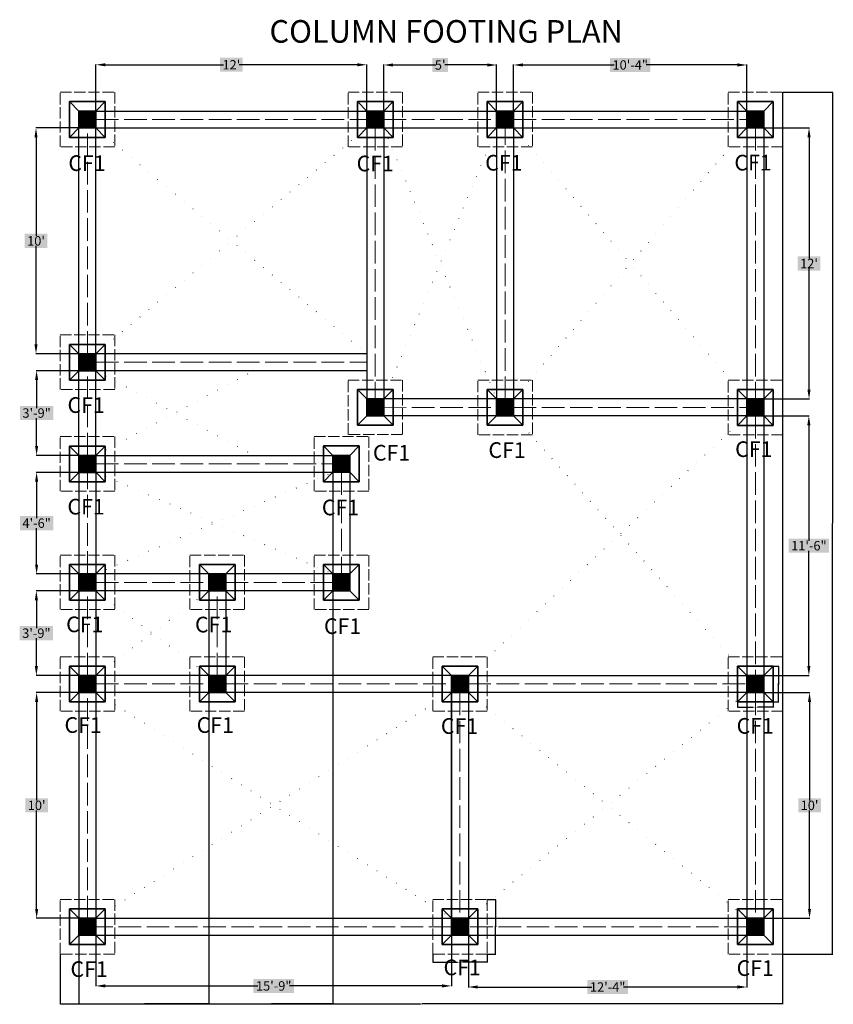
# Model space of a CAD drawing. Units: inches. Extents: x -128 to 854, y -395 to 398.
# Tile 61 of 61: x 395 to 828, y -125 to 398. Entities that reach past the tile are written whole.
import ezdxf

# ---------------------------------------------------------------- set-up
doc = ezdxf.new("R2010")
doc.units = ezdxf.units.IN
doc.header["$MEASUREMENT"] = 0
doc.linetypes.add('ACAD_ISO02W100', pattern=[15, 12, -3])
doc.linetypes.add('ACAD_ISO07W100', pattern=[3, 0, -3])
for name, color, linetype, lineweight in [('A-ANNO-DIMS', 2, 'Continuous', 18), ('A-ANNO-TITL', 7, 'Continuous', 25), ('S-ANNO-DIMS', 2, 'Continuous', 18), ('S-ANNO-TEXT', 7, 'Continuous', 18), ('S-BEAM', 152, 'Continuous', 30), ('S-BEAM-CNTR', 6, 'ACAD_ISO02W100', 13), ('S-COLS', 7, 'Continuous', 35), ('S-COLS-PATT', 8, 'Continuous', 13), ('S-FNDN', 2, 'Continuous', 35), ('S-FNDN-DIAG', 252, 'ACAD_ISO07W100', 13), ('S-FNDN-HIDN', 3, 'ACAD_ISO02W100', 18)]:
    doc.layers.add(name, color=color, linetype=linetype, lineweight=lineweight)
doc.styles.get("Standard").update_dxf_attribs({"font": 'arial.ttf'})
doc.dimstyles.get("Standard").update_dxf_attribs({"dimtxt": 0.18, "dimasz": 0.18, "dimexe": 0.18, "dimexo": 0.0625, "dimgap": 0.09, "dimtad": 0, "dimtih": 1, "dimtoh": 1, "dimdec": 1, "dimzin": 0, "dimdsep": 46, "dimlunit": 4, "dimtxsty": 'Standard', "dimcen": 0.09, "dimclrd": 1, "dimclre": 2, "dimclrt": 6, "dimadec": 0, "dimazin": 0, "dimtfac": 1, "dimtdec": 1, "dimtofl": 0, "dimtmove": 0, "dimatfit": 3, "dimfxl": 1, "dimtfill": 2, "dimtfillclr": 3, "dimtolj": 1, "dimtzin": 0, "dimarcsym": 0})

# ---------------------------------------------------------------- blocks, each defined once
blk = doc.blocks.new('*D16')
at = {"layer": 'Defpoints', "color": 0, "transparency": 16777216}
for p in [(435.64, -79.2), (624.64, -79.2), (624.64, -115.16)]:
    blk.add_point(p, dxfattribs=at)
at = {"layer": 'S-ANNO-DIMS', "color": 0, "lineweight": -2, "transparency": 16777216}
for p, q in [((435.64, -79.27), (435.64, -115.34)), ((624.64, -79.27), (624.64, -115.34)), ((440.64, -115.16), (521.69, -115.16)), ((619.64, -115.16), (538.58, -115.16))]:
    blk.add_line(p, q, dxfattribs=at)
at = {"layer": 'S-ANNO-DIMS', "color": 0, "transparency": 16777216}
for points in [[(440.64, -114.33), (440.64, -116), (435.64, -115.16)], [(619.64, -114.33), (619.64, -116), (624.64, -115.16)]]:
    blk.add_solid(points, dxfattribs=at)
at = {"layer": 'S-ANNO-DIMS', "color": 0, "transparency": 16777216, "insert": (530.14, -115.16), "char_height": 5, "attachment_point": 5, "bg_fill": 1, "box_fill_scale": 1.25, "bg_fill_color": 3, "bg_fill_transparency": 0}
blk.add_mtext('\\A1;15\'-9"', dxfattribs=at)
blk = doc.blocks.new('*D17')
at = {"layer": 'Defpoints', "color": 0, "transparency": 16777216}
for p in [(633.64, -79.2), (781.64, -79.2), (781.64, -115.74)]:
    blk.add_point(p, dxfattribs=at)
at = {"layer": 'S-ANNO-DIMS', "color": 0, "lineweight": -2, "transparency": 16777216}
for p, q in [((633.64, -79.27), (633.64, -115.92)), ((781.64, -79.27), (781.64, -115.92)), ((638.64, -115.74), (699.19, -115.74)), ((776.64, -115.74), (716.08, -115.74))]:
    blk.add_line(p, q, dxfattribs=at)
at = {"layer": 'S-ANNO-DIMS', "color": 0, "transparency": 16777216}
for points in [[(638.64, -114.9), (638.64, -116.57), (633.64, -115.74)], [(776.64, -114.9), (776.64, -116.57), (781.64, -115.74)]]:
    blk.add_solid(points, dxfattribs=at)
at = {"layer": 'S-ANNO-DIMS', "color": 0, "transparency": 16777216, "insert": (707.64, -115.74), "char_height": 5, "attachment_point": 5, "bg_fill": 1, "box_fill_scale": 1.25, "bg_fill_color": 3, "bg_fill_transparency": 0}
blk.add_mtext('\\A1;12\'-4"', dxfattribs=at)
blk = doc.blocks.new('*D18')
at = {"layer": 'Defpoints', "color": 0, "transparency": 16777216}
for p in [(781.64, 40.8), (814.94, 40.8), (781.64, -79.2)]:
    blk.add_point(p, dxfattribs=at)
at = {"layer": 'S-ANNO-DIMS', "color": 0, "lineweight": -2, "transparency": 16777216}
for p, q in [((781.7, 40.8), (815.12, 40.8)), ((814.94, 35.8), (814.94, -16.56)), ((814.94, -74.2), (814.94, -21.85)), ((781.7, -79.2), (815.12, -79.2))]:
    blk.add_line(p, q, dxfattribs=at)
at = {"layer": 'S-ANNO-DIMS', "color": 0, "transparency": 16777216}
for points in [[(814.1, 35.8), (815.77, 35.8), (814.94, 40.8)], [(814.1, -74.2), (815.77, -74.2), (814.94, -79.2)]]:
    blk.add_solid(points, dxfattribs=at)
at = {"layer": 'S-ANNO-DIMS', "color": 0, "transparency": 16777216, "insert": (814.94, -19.2), "char_height": 5, "attachment_point": 5, "bg_fill": 1, "box_fill_scale": 1.25, "bg_fill_color": 3, "bg_fill_transparency": 0}
blk.add_mtext("\\A1;10'", dxfattribs=at)
blk = doc.blocks.new('*D19')
at = {"layer": 'Defpoints', "color": 0, "transparency": 16777216}
for p in [(781.64, 187.8), (814.59, 187.8), (781.64, 49.8)]:
    blk.add_point(p, dxfattribs=at)
at = {"layer": 'S-ANNO-DIMS', "color": 0, "lineweight": -2, "transparency": 16777216}
for p, q in [((781.7, 187.8), (814.77, 187.8)), ((781.7, 49.8), (814.77, 49.8))]:
    blk.add_line(p, q, dxfattribs=at)
at = {"layer": 'S-ANNO-DIMS', "color": 0, "lineweight": -3, "transparency": 16777216}
for p, q in [((814.59, 182.8), (814.59, 121.44)), ((814.59, 54.8), (814.59, 116.15))]:
    blk.add_line(p, q, dxfattribs=at)
at = {"layer": 'S-ANNO-DIMS', "color": 0, "transparency": 16777216}
for points in [[(813.76, 182.8), (815.42, 182.8), (814.59, 187.8)], [(813.76, 54.8), (815.42, 54.8), (814.59, 49.8)]]:
    blk.add_solid(points, dxfattribs=at)
at = {"layer": 'S-ANNO-DIMS', "color": 0, "transparency": 16777216, "insert": (814.59, 118.8), "char_height": 5, "attachment_point": 5, "bg_fill": 1, "box_fill_scale": 1.25, "bg_fill_color": 3, "bg_fill_transparency": 0}
blk.add_mtext('\\A1;11\'-6"', dxfattribs=at)
blk = doc.blocks.new('*D20')
at = {"layer": 'Defpoints', "color": 0, "transparency": 16777216}
for p in [(781.64, 340.8), (814.67, 340.8), (781.64, 196.76)]:
    blk.add_point(p, dxfattribs=at)
at = {"layer": 'S-ANNO-DIMS', "color": 0, "lineweight": -2, "transparency": 16777216}
for p, q in [((781.7, 340.8), (814.85, 340.8)), ((814.67, 335.8), (814.67, 271.38)), ((814.67, 201.76), (814.67, 266.18)), ((781.7, 196.76), (814.85, 196.76))]:
    blk.add_line(p, q, dxfattribs=at)
at = {"layer": 'S-ANNO-DIMS', "color": 0, "transparency": 16777216}
for points in [[(813.83, 335.8), (815.5, 335.8), (814.67, 340.8)], [(813.83, 201.76), (815.5, 201.76), (814.67, 196.76)]]:
    blk.add_solid(points, dxfattribs=at)
at = {"layer": 'S-ANNO-DIMS', "color": 0, "transparency": 16777216, "insert": (814.67, 268.78), "char_height": 5, "attachment_point": 5, "bg_fill": 1, "box_fill_scale": 1.25, "bg_fill_color": 3, "bg_fill_transparency": 0}
blk.add_mtext("\\A1;12'", dxfattribs=at)
blk = doc.blocks.new('*D21')
at = {"layer": 'Defpoints', "color": 0, "transparency": 16777216}
for p in [(781.64, 374.28), (657.64, 340.8), (781.64, 340.8)]:
    blk.add_point(p, dxfattribs=at)
at = {"layer": 'S-ANNO-DIMS', "color": 0, "lineweight": -2, "transparency": 16777216}
for p, q in [((657.64, 340.86), (657.64, 374.46)), ((662.64, 374.28), (711.19, 374.28)), ((776.64, 374.28), (728.08, 374.28)), ((781.64, 340.86), (781.64, 374.46))]:
    blk.add_line(p, q, dxfattribs=at)
at = {"layer": 'S-ANNO-DIMS', "color": 0, "transparency": 16777216}
for points in [[(662.64, 375.12), (662.64, 373.45), (657.64, 374.28)], [(776.64, 375.12), (776.64, 373.45), (781.64, 374.28)]]:
    blk.add_solid(points, dxfattribs=at)
at = {"layer": 'S-ANNO-DIMS', "color": 0, "transparency": 16777216, "insert": (719.64, 374.28), "char_height": 5, "attachment_point": 5, "bg_fill": 1, "box_fill_scale": 1.25, "bg_fill_color": 3, "bg_fill_transparency": 0}
blk.add_mtext('\\A1;10\'-4"', dxfattribs=at)
blk = doc.blocks.new('*D22')
at = {"layer": 'Defpoints', "color": 0, "transparency": 16777216}
for p in [(648.64, 374.27), (588.64, 340.8), (648.64, 340.8)]:
    blk.add_point(p, dxfattribs=at)
at = {"layer": 'S-ANNO-DIMS', "color": 0, "lineweight": -2, "transparency": 16777216}
for p, q in [((588.64, 340.86), (588.64, 374.45)), ((593.64, 374.27), (616.25, 374.27)), ((643.64, 374.27), (621.03, 374.27)), ((648.64, 340.86), (648.64, 374.45))]:
    blk.add_line(p, q, dxfattribs=at)
at = {"layer": 'S-ANNO-DIMS', "color": 0, "transparency": 16777216}
for points in [[(593.64, 375.1), (593.64, 373.43), (588.64, 374.27)], [(643.64, 375.1), (643.64, 373.43), (648.64, 374.27)]]:
    blk.add_solid(points, dxfattribs=at)
at = {"layer": 'S-ANNO-DIMS', "color": 0, "transparency": 16777216, "insert": (618.64, 374.27), "char_height": 5, "attachment_point": 5, "bg_fill": 1, "box_fill_scale": 1.25, "bg_fill_color": 3, "bg_fill_transparency": 0}
blk.add_mtext("\\A1;5'", dxfattribs=at)
blk = doc.blocks.new('*D23')
at = {"layer": 'Defpoints', "color": 0, "transparency": 16777216}
for p in [(579.64, 374.38), (435.64, 340.8), (579.64, 340.8)]:
    blk.add_point(p, dxfattribs=at)
at = {"layer": 'S-ANNO-DIMS', "color": 0, "lineweight": -2, "transparency": 16777216}
for p, q in [((435.64, 340.86), (435.64, 374.56)), ((440.64, 374.38), (503.54, 374.38)), ((574.64, 374.38), (511.73, 374.38)), ((579.64, 340.86), (579.64, 374.56))]:
    blk.add_line(p, q, dxfattribs=at)
at = {"layer": 'S-ANNO-DIMS', "color": 0, "transparency": 16777216}
for points in [[(440.64, 375.21), (440.64, 373.55), (435.64, 374.38)], [(574.64, 375.21), (574.64, 373.55), (579.64, 374.38)]]:
    blk.add_solid(points, dxfattribs=at)
at = {"layer": 'S-ANNO-DIMS', "color": 0, "transparency": 16777216, "insert": (507.64, 374.38), "char_height": 5, "attachment_point": 5, "bg_fill": 1, "box_fill_scale": 1.25, "bg_fill_color": 3, "bg_fill_transparency": 0}
blk.add_mtext("\\A1;12'", dxfattribs=at)
blk = doc.blocks.new('*D24')
at = {"layer": 'Defpoints', "color": 0, "transparency": 16777216}
for p in [(435.64, 340.8), (403.82, 220.8), (435.64, 220.8)]:
    blk.add_point(p, dxfattribs=at)
at = {"layer": 'S-ANNO-DIMS', "color": 0, "lineweight": -2, "transparency": 16777216}
for p, q in [((435.57, 340.8), (403.64, 340.8)), ((403.82, 335.8), (403.82, 283.44)), ((403.82, 225.8), (403.82, 278.15)), ((435.57, 220.8), (403.64, 220.8))]:
    blk.add_line(p, q, dxfattribs=at)
at = {"layer": 'S-ANNO-DIMS', "color": 0, "transparency": 16777216}
for points in [[(402.99, 335.8), (404.65, 335.8), (403.82, 340.8)], [(402.99, 225.8), (404.65, 225.8), (403.82, 220.8)]]:
    blk.add_solid(points, dxfattribs=at)
at = {"layer": 'S-ANNO-DIMS', "color": 0, "transparency": 16777216, "insert": (403.82, 280.8), "char_height": 5, "attachment_point": 5, "bg_fill": 1, "box_fill_scale": 1.25, "bg_fill_color": 3, "bg_fill_transparency": 0}
blk.add_mtext("\\A1;10'", dxfattribs=at)
blk = doc.blocks.new('*D25')
at = {"layer": 'Defpoints', "color": 0, "transparency": 16777216}
for p in [(435.64, 211.8), (404.14, 166.8), (435.64, 166.8)]:
    blk.add_point(p, dxfattribs=at)
at = {"layer": 'S-ANNO-DIMS', "color": 0, "lineweight": -2, "transparency": 16777216}
for p, q in [((435.57, 211.8), (403.96, 211.8)), ((404.14, 206.8), (404.14, 191.94)), ((404.14, 171.8), (404.14, 186.65)), ((435.57, 166.8), (403.96, 166.8))]:
    blk.add_line(p, q, dxfattribs=at)
at = {"layer": 'S-ANNO-DIMS', "color": 0, "transparency": 16777216}
for points in [[(403.3, 206.8), (404.97, 206.8), (404.14, 211.8)], [(403.3, 171.8), (404.97, 171.8), (404.14, 166.8)]]:
    blk.add_solid(points, dxfattribs=at)
at = {"layer": 'S-ANNO-DIMS', "color": 0, "transparency": 16777216, "insert": (404.14, 189.3), "char_height": 5, "attachment_point": 5, "bg_fill": 1, "box_fill_scale": 1.25, "bg_fill_color": 3, "bg_fill_transparency": 0}
blk.add_mtext('\\A1;3\'-9"', dxfattribs=at)
blk = doc.blocks.new('*D26')
at = {"layer": 'Defpoints', "color": 0, "transparency": 16777216}
for p in [(435.64, 157.76), (404.15, 103.8), (435.64, 103.8)]:
    blk.add_point(p, dxfattribs=at)
at = {"layer": 'S-ANNO-DIMS', "color": 0, "lineweight": -2, "transparency": 16777216}
for p, q in [((435.57, 157.76), (403.97, 157.76)), ((404.15, 152.76), (404.15, 133.42)), ((404.15, 108.8), (404.15, 128.14)), ((435.57, 103.8), (403.97, 103.8))]:
    blk.add_line(p, q, dxfattribs=at)
at = {"layer": 'S-ANNO-DIMS', "color": 0, "transparency": 16777216}
for points in [[(403.31, 152.76), (404.98, 152.76), (404.15, 157.76)], [(403.31, 108.8), (404.98, 108.8), (404.15, 103.8)]]:
    blk.add_solid(points, dxfattribs=at)
at = {"layer": 'S-ANNO-DIMS', "color": 0, "transparency": 16777216, "insert": (404.15, 130.78), "char_height": 5, "attachment_point": 5, "bg_fill": 1, "box_fill_scale": 1.25, "bg_fill_color": 3, "bg_fill_transparency": 0}
blk.add_mtext('\\A1;4\'-6"', dxfattribs=at)
blk = doc.blocks.new('*D27')
at = {"layer": 'Defpoints', "color": 0, "transparency": 16777216}
for p in [(435.64, 94.8), (404.01, 49.8), (435.64, 49.8)]:
    blk.add_point(p, dxfattribs=at)
at = {"layer": 'S-ANNO-DIMS', "color": 0, "lineweight": -2, "transparency": 16777216}
for p, q in [((435.57, 94.8), (403.83, 94.8)), ((404.01, 89.8), (404.01, 74.94)), ((404.01, 54.8), (404.01, 69.65)), ((435.57, 49.8), (403.83, 49.8))]:
    blk.add_line(p, q, dxfattribs=at)
at = {"layer": 'S-ANNO-DIMS', "color": 0, "transparency": 16777216}
for points in [[(403.17, 89.8), (404.84, 89.8), (404.01, 94.8)], [(403.17, 54.8), (404.84, 54.8), (404.01, 49.8)]]:
    blk.add_solid(points, dxfattribs=at)
at = {"layer": 'S-ANNO-DIMS', "color": 0, "transparency": 16777216, "insert": (404.01, 72.3), "char_height": 5, "attachment_point": 5, "bg_fill": 1, "box_fill_scale": 1.25, "bg_fill_color": 3, "bg_fill_transparency": 0}
blk.add_mtext('\\A1;3\'-9"', dxfattribs=at)
blk = doc.blocks.new('*D28')
at = {"layer": 'Defpoints', "color": 0, "transparency": 16777216}
for p in [(404.16, 40.8), (435.64, 40.8), (435.64, -79.2)]:
    blk.add_point(p, dxfattribs=at)
at = {"layer": 'S-ANNO-DIMS', "color": 0, "lineweight": -2, "transparency": 16777216}
for p, q in [((435.57, 40.8), (403.98, 40.8)), ((404.16, 35.8), (404.16, -16.56)), ((404.16, -74.2), (404.16, -21.85)), ((435.57, -79.2), (403.98, -79.2))]:
    blk.add_line(p, q, dxfattribs=at)
at = {"layer": 'S-ANNO-DIMS', "color": 0, "transparency": 16777216}
for points in [[(403.33, 35.8), (405, 35.8), (404.16, 40.8)], [(403.33, -74.2), (405, -74.2), (404.16, -79.2)]]:
    blk.add_solid(points, dxfattribs=at)
at = {"layer": 'S-ANNO-DIMS', "color": 0, "transparency": 16777216, "insert": (404.16, -19.2), "char_height": 5, "attachment_point": 5, "bg_fill": 1, "box_fill_scale": 1.25, "bg_fill_color": 3, "bg_fill_transparency": 0}
blk.add_mtext("\\A1;10'", dxfattribs=at)
blk = doc.blocks.new('CF1-BASE-29IN')
at = {"ltscale": 0.5}
for p, q in [((0, 29), (29, 29)), ((0, 0), (0, 29)), ((29, 29), (29, 0)), ((29, 0), (0, 0))]:
    blk.add_line(p, q, dxfattribs=at)
blk = doc.blocks.new('CF1-PAD-19IN')
for p, q in [((0, 19), (19, 19)), ((0, 0), (0, 19)), ((19, 19), (19, 0)), ((19, 0), (0, 0))]:
    blk.add_line(p, q)
blk = doc.blocks.new('*D67')
at = {"layer": 'A-ANNO-DIMS', "color": 2, "lineweight": -2, "transparency": 16777216}
for p, q in [((614.64, -98.27), (614.64, -102.73)), ((643.64, -98.27), (643.64, -102.73))]:
    blk.add_line(p, q, dxfattribs=at)
at = {"layer": 'A-ANNO-DIMS', "color": 1, "lineweight": -2, "transparency": 16777216}
for p, q in [((614.82, -102.55), (627.86, -102.55)), ((643.46, -102.55), (630.42, -102.55))]:
    blk.add_line(p, q, dxfattribs=at)
at = {"layer": 'A-ANNO-DIMS', "color": 1, "transparency": 16777216}
for points in [[(614.82, -102.52), (614.82, -102.58), (614.64, -102.55)], [(643.46, -102.52), (643.46, -102.58), (643.64, -102.55)]]:
    blk.add_solid(points, dxfattribs=at)
at = {"layer": 'Defpoints', "color": 0, "transparency": 16777216}
for p in [(614.64, -98.2), (643.64, -98.2), (643.64, -102.55)]:
    blk.add_point(p, dxfattribs=at)
at = {"layer": 'A-ANNO-DIMS', "color": 6, "transparency": 16777216, "insert": (629.14, -102.55), "char_height": 0.18, "attachment_point": 5, "bg_fill": 1, "box_fill_scale": 1.25, "bg_fill_color": 3, "bg_fill_transparency": 0}
blk.add_mtext('\\A1;CF1 BASE 2\'-5" TYP.', dxfattribs=at)
blk = doc.blocks.new('*D68')
at = {"layer": 'A-ANNO-DIMS', "color": 2, "lineweight": -2, "transparency": 16777216}
for p, q in [((643.7, -69.2), (648.17, -69.2)), ((643.7, -98.2), (648.17, -98.2))]:
    blk.add_line(p, q, dxfattribs=at)
at = {"layer": 'A-ANNO-DIMS', "color": 1, "lineweight": -2, "transparency": 16777216}
for p, q in [((647.99, -69.38), (647.99, -83.52)), ((647.99, -98.02), (647.99, -83.88))]:
    blk.add_line(p, q, dxfattribs=at)
at = {"layer": 'A-ANNO-DIMS', "color": 1, "transparency": 16777216}
for points in [[(647.96, -69.38), (648.02, -69.38), (647.99, -69.2)], [(647.96, -98.02), (648.02, -98.02), (647.99, -98.2)]]:
    blk.add_solid(points, dxfattribs=at)
at = {"layer": 'Defpoints', "color": 0, "transparency": 16777216}
for p in [(643.64, -69.2), (647.99, -69.2), (643.64, -98.2)]:
    blk.add_point(p, dxfattribs=at)
at = {"layer": 'A-ANNO-DIMS', "color": 6, "transparency": 16777216, "insert": (647.99, -83.7), "char_height": 0.18, "attachment_point": 5, "bg_fill": 1, "box_fill_scale": 1.25, "bg_fill_color": 3, "bg_fill_transparency": 0}
blk.add_mtext('\\A1;2\'-5" TYP.', dxfattribs=at)
blk = doc.blocks.new('*D69')
at = {"layer": 'A-ANNO-DIMS', "color": 2, "lineweight": -2, "transparency": 16777216}
for p, q in [((776.64, 35.73), (776.64, 32.77)), ((795.64, 35.73), (795.64, 32.77))]:
    blk.add_line(p, q, dxfattribs=at)
at = {"layer": 'A-ANNO-DIMS', "color": 1, "lineweight": -2, "transparency": 16777216}
for p, q in [((776.82, 32.95), (784.93, 32.95)), ((795.46, 32.95), (787.34, 32.95))]:
    blk.add_line(p, q, dxfattribs=at)
at = {"layer": 'A-ANNO-DIMS', "color": 1, "transparency": 16777216}
for points in [[(776.82, 32.98), (776.82, 32.92), (776.64, 32.95)], [(795.46, 32.98), (795.46, 32.92), (795.64, 32.95)]]:
    blk.add_solid(points, dxfattribs=at)
at = {"layer": 'Defpoints', "color": 0, "transparency": 16777216}
for p in [(776.64, 35.8), (795.64, 35.8), (795.64, 32.95)]:
    blk.add_point(p, dxfattribs=at)
at = {"layer": 'A-ANNO-DIMS', "color": 6, "transparency": 16777216, "insert": (786.14, 32.95), "char_height": 0.18, "attachment_point": 5, "bg_fill": 1, "box_fill_scale": 1.25, "bg_fill_color": 3, "bg_fill_transparency": 0}
blk.add_mtext('\\A1;CF1 PAD 1\'-7" TYP.', dxfattribs=at)
blk = doc.blocks.new('*D70')
at = {"layer": 'A-ANNO-DIMS', "color": 2, "lineweight": -2, "transparency": 16777216}
for p, q in [((795.7, 54.8), (798.67, 54.8)), ((795.7, 35.8), (798.67, 35.8))]:
    blk.add_line(p, q, dxfattribs=at)
at = {"layer": 'A-ANNO-DIMS', "color": 1, "lineweight": -2, "transparency": 16777216}
for p, q in [((798.49, 54.62), (798.49, 45.48)), ((798.49, 35.98), (798.49, 45.12))]:
    blk.add_line(p, q, dxfattribs=at)
at = {"layer": 'A-ANNO-DIMS', "color": 1, "transparency": 16777216}
for points in [[(798.46, 54.62), (798.52, 54.62), (798.49, 54.8)], [(798.46, 35.98), (798.52, 35.98), (798.49, 35.8)]]:
    blk.add_solid(points, dxfattribs=at)
at = {"layer": 'Defpoints', "color": 0, "transparency": 16777216}
for p in [(795.64, 54.8), (798.49, 54.8), (795.64, 35.8)]:
    blk.add_point(p, dxfattribs=at)
at = {"layer": 'A-ANNO-DIMS', "color": 6, "transparency": 16777216, "insert": (798.49, 45.3), "char_height": 0.18, "attachment_point": 5, "bg_fill": 1, "box_fill_scale": 1.25, "bg_fill_color": 3, "bg_fill_transparency": 0}
blk.add_mtext('\\A1;1\'-7" TYP.', dxfattribs=at)
blk = doc.blocks.new('*D115')
at = {"layer": 'A-ANNO-DIMS', "color": 2, "lineweight": -2, "transparency": 16777216}
for p, q in [((800.64, 359.73), (800.64, -124.93)), ((416.64, -98.27), (416.64, -124.93))]:
    blk.add_line(p, q, dxfattribs=at)
at = {"layer": 'A-ANNO-DIMS', "color": 1, "lineweight": -2, "transparency": 16777216}
for p, q in [((416.82, -124.75), (608.24, -124.75)), ((800.46, -124.75), (609.04, -124.75))]:
    blk.add_line(p, q, dxfattribs=at)
at = {"layer": 'A-ANNO-DIMS', "color": 1, "transparency": 16777216}
for points in [[(416.82, -124.72), (416.82, -124.78), (416.64, -124.75)], [(800.46, -124.72), (800.46, -124.78), (800.64, -124.75)]]:
    blk.add_solid(points, dxfattribs=at)
at = {"layer": 'Defpoints', "color": 0, "transparency": 16777216}
for p in [(800.64, 359.8), (416.64, -98.2), (800.64, -124.75)]:
    blk.add_point(p, dxfattribs=at)
at = {"layer": 'A-ANNO-DIMS', "color": 6, "transparency": 16777216, "insert": (608.64, -124.75), "char_height": 0.18, "attachment_point": 5, "bg_fill": 1, "box_fill_scale": 1.25, "bg_fill_color": 3, "bg_fill_transparency": 0}
blk.add_mtext('\\A1;32\'-0"', dxfattribs=at)
blk = doc.blocks.new('*D116')
at = {"layer": 'A-ANNO-DIMS', "color": 2, "lineweight": -2, "transparency": 16777216}
for p, q in [((800.7, 359.8), (827.37, 359.8)), ((800.7, -98.2), (827.37, -98.2))]:
    blk.add_line(p, q, dxfattribs=at)
at = {"layer": 'A-ANNO-DIMS', "color": 1, "lineweight": -2, "transparency": 16777216}
for p, q in [((827.19, 359.62), (827.19, 130.98)), ((827.19, -98.02), (827.19, 130.62))]:
    blk.add_line(p, q, dxfattribs=at)
at = {"layer": 'A-ANNO-DIMS', "color": 1, "transparency": 16777216}
for points in [[(827.16, 359.62), (827.22, 359.62), (827.19, 359.8)], [(827.16, -98.02), (827.22, -98.02), (827.19, -98.2)]]:
    blk.add_solid(points, dxfattribs=at)
at = {"layer": 'Defpoints', "color": 0, "transparency": 16777216}
for p in [(800.64, 359.8), (827.19, 359.8), (800.64, -98.2)]:
    blk.add_point(p, dxfattribs=at)
at = {"layer": 'A-ANNO-DIMS', "color": 6, "transparency": 16777216, "insert": (827.19, 130.8), "char_height": 0.18, "attachment_point": 5, "bg_fill": 1, "box_fill_scale": 1.25, "bg_fill_color": 3, "bg_fill_transparency": 0}
blk.add_mtext('\\A1;38\'-2"', dxfattribs=at)
blk = doc.blocks.new('*D117')
at = {"layer": 'A-ANNO-DIMS', "color": 2, "lineweight": -2, "transparency": 16777216}
for p, q in [((426.64, 103.73), (426.64, -124.93)), ((495.64, 103.73), (495.64, -124.93))]:
    blk.add_line(p, q, dxfattribs=at)
at = {"layer": 'A-ANNO-DIMS', "color": 1, "lineweight": -2, "transparency": 16777216}
for p, q in [((426.82, -124.75), (460.81, -124.75)), ((495.46, -124.75), (461.47, -124.75))]:
    blk.add_line(p, q, dxfattribs=at)
at = {"layer": 'A-ANNO-DIMS', "color": 1, "transparency": 16777216}
for points in [[(426.82, -124.72), (426.82, -124.78), (426.64, -124.75)], [(495.46, -124.72), (495.46, -124.78), (495.64, -124.75)]]:
    blk.add_solid(points, dxfattribs=at)
at = {"layer": 'Defpoints', "color": 0, "transparency": 16777216}
for p in [(426.64, 103.8), (495.64, 103.8), (495.64, -124.75)]:
    blk.add_point(p, dxfattribs=at)
at = {"layer": 'A-ANNO-DIMS', "color": 6, "transparency": 16777216, "insert": (461.14, -124.75), "char_height": 0.18, "attachment_point": 5, "bg_fill": 1, "box_fill_scale": 1.25, "bg_fill_color": 3, "bg_fill_transparency": 0}
blk.add_mtext('\\A1;5\'-9"', dxfattribs=at)
blk = doc.blocks.new('*D118')
at = {"layer": 'A-ANNO-DIMS', "color": 2, "lineweight": -2, "transparency": 16777216}
for p, q in [((495.64, 103.73), (495.64, -124.93)), ((561.64, 103.73), (561.64, -124.93))]:
    blk.add_line(p, q, dxfattribs=at)
at = {"layer": 'A-ANNO-DIMS', "color": 1, "lineweight": -2, "transparency": 16777216}
for p, q in [((495.82, -124.75), (528.31, -124.75)), ((561.46, -124.75), (528.97, -124.75))]:
    blk.add_line(p, q, dxfattribs=at)
at = {"layer": 'A-ANNO-DIMS', "color": 1, "transparency": 16777216}
for points in [[(495.82, -124.72), (495.82, -124.78), (495.64, -124.75)], [(561.46, -124.72), (561.46, -124.78), (561.64, -124.75)]]:
    blk.add_solid(points, dxfattribs=at)
at = {"layer": 'Defpoints', "color": 0, "transparency": 16777216}
for p in [(495.64, 103.8), (561.64, 103.8), (561.64, -124.75)]:
    blk.add_point(p, dxfattribs=at)
at = {"layer": 'A-ANNO-DIMS', "color": 6, "transparency": 16777216, "insert": (528.64, -124.75), "char_height": 0.18, "attachment_point": 5, "bg_fill": 1, "box_fill_scale": 1.25, "bg_fill_color": 3, "bg_fill_transparency": 0}
blk.add_mtext('\\A1;5\'-6"', dxfattribs=at)

msp = doc.modelspace()

# ---------------------------------------------------------------- hatches: boundary and pattern name
at = {"layer": 'S-COLS-PATT'}
h = msp.add_hatch(dxfattribs=at)
h.set_pattern_fill('ANSI31', color=256)
h.paths.add_polyline_path([(435.64, 349.8), (426.64, 349.8), (426.64, 340.8), (435.64, 340.8)])
h.paths.add_polyline_path([(588.64, 349.8), (579.64, 349.8), (579.64, 340.8), (588.64, 340.8)])
h.paths.add_polyline_path([(657.64, 349.8), (648.64, 349.8), (648.64, 340.8), (657.64, 340.8)])
h.paths.add_polyline_path([(790.64, 349.8), (781.64, 349.8), (781.64, 340.8), (790.64, 340.8)])
h.paths.add_polyline_path([(435.64, 220.8), (426.64, 220.8), (426.64, 211.8), (435.64, 211.8)])
h.paths.add_polyline_path([(588.64, 196.8), (579.64, 196.8), (579.64, 187.83), (588.64, 187.83)])
h.paths.add_polyline_path([(657.64, 196.8), (648.64, 196.8), (648.64, 187.8), (657.64, 187.8)])
h.paths.add_polyline_path([(790.64, 196.76), (781.64, 196.76), (781.64, 187.76), (790.64, 187.76)])
h.paths.add_polyline_path([(435.64, 166.76), (426.64, 166.76), (426.64, 157.76), (435.64, 157.76)])
h.paths.add_polyline_path([(570.64, 166.8), (561.64, 166.8), (561.64, 157.8), (570.64, 157.8)])
h.paths.add_polyline_path([(435.64, 103.8), (426.64, 103.8), (426.64, 94.8), (435.64, 94.8)])
h.paths.add_polyline_path([(504.64, 103.8), (495.64, 103.8), (495.64, 94.8), (504.64, 94.8)])
h.paths.add_polyline_path([(570.64, 103.8), (561.64, 103.8), (561.64, 94.8), (570.64, 94.8)])
h.paths.add_polyline_path([(435.64, 49.8), (426.64, 49.8), (426.64, 40.8), (435.64, 40.8)])
h.paths.add_polyline_path([(504.64, 49.8), (495.64, 49.8), (495.64, 40.8), (504.64, 40.8)])
h.paths.add_polyline_path([(633.64, 49.8), (624.64, 49.8), (624.64, 40.8), (633.64, 40.8)])
h.paths.add_polyline_path([(790.64, 49.8), (781.64, 49.8), (781.64, 40.8), (790.64, 40.8)])
h.paths.add_polyline_path([(435.64, -79.2), (426.64, -79.2), (426.64, -88.2), (435.64, -88.2)])
h.paths.add_polyline_path([(633.64, -79.2), (624.64, -79.2), (624.64, -88.2), (633.64, -88.2)])
h.paths.add_polyline_path([(790.64, -79.2), (781.64, -79.2), (781.64, -88.2), (790.64, -88.2)])

# ---------------------------------------------------------------- linework, layer by layer
at = {"layer": 'S-BEAM'}
for p, q in [((426.64, 162.3), (426.64, 349.8)), ((426.64, 349.8), (790.64, 349.8)), ((790.64, 349.8), (790.64, -88.2)), ((435.64, 220.8), (435.64, 340.8)), ((435.64, 340.8), (579.64, 340.8)), ((579.64, 340.8), (579.64, 187.8)), ((588.64, 340.8), (588.64, 187.8)), ((588.64, 340.8), (648.64, 340.8)), ((648.64, 340.8), (648.64, 220.8)), ((648.64, 340.8), (648.64, 196.83)), ((657.64, 340.8), (657.64, 196.8)), ((657.64, 340.8), (781.64, 340.8)), ((781.64, 340.8), (781.64, 196.8)), ((579.64, 220.8), (435.64, 220.8)), ((579.64, 211.8), (426.64, 211.8)), ((435.64, 166.8), (435.64, 211.8)), ((781.64, 196.8), (579.64, 196.8)), ((781.64, 187.8), (579.64, 187.8)), ((781.64, 187.8), (781.64, 73.8)), ((426.64, 166.8), (570.64, 166.8)), ((570.64, 166.8), (570.64, 94.8)), ((426.64, 161.98), (426.64, 94.8)), ((435.64, 157.8), (435.64, 103.8)), ((435.64, 157.8), (561.64, 157.8)), ((561.64, 157.8), (561.64, 103.8)), ((435.64, 103.8), (435.64, 49.8)), ((561.64, 103.8), (435.64, 103.8)), ((426.64, 94.8), (426.64, 40.8)), ((570.64, 94.8), (435.64, 94.8)), ((495.64, 94.8), (495.64, 49.8)), ((504.64, 94.8), (504.64, 49.8)), ((781.64, 84.8), (781.64, -79.2)), ((495.64, 49.8), (435.64, 49.8)), ((633.64, 49.8), (504.64, 49.8)), ((633.64, 49.8), (633.64, -79.2)), ((633.64, 49.8), (790.64, 49.8)), ((426.64, 40.8), (426.64, -88.2)), ((519.64, 40.8), (435.64, 40.8)), ((435.64, 40.8), (435.64, -79.2)), ((790.64, 40.8), (495.64, 40.8)), ((624.64, -79.2), (624.64, 40.8)), ((624.64, 40.8), (624.64, -79.2)), ((435.64, -79.2), (561.64, -79.2)), ((559.66, -79.2), (624.64, -79.2)), ((633.64, -79.2), (781.64, -79.2)), ((426.64, -88.2), (528.64, -88.2)), ((528.64, -88.2), (633.64, -88.2)), ((633.64, -88.2), (790.64, -88.2))]:
    msp.add_line(p, q, dxfattribs=at)
at = {"layer": 'S-BEAM-CNTR'}
for p, q in [((431.14, 220.8), (431.14, 340.8)), ((435.64, 345.3), (579.64, 345.3)), ((584.14, 340.8), (584.14, 196.8)), ((588.64, 345.3), (648.64, 345.3)), ((653.14, 196.8), (653.14, 340.8)), ((657.64, 345.3), (781.64, 345.3)), ((786.14, 340.8), (786.14, 196.8)), ((435.64, 216.3), (579.64, 216.3)), ((431.14, 166.8), (431.14, 211.8)), ((588.64, 192.33), (648.64, 192.3)), ((657.64, 192.3), (781.64, 192.28)), ((584.14, 187.83), (584.14, 187.8)), ((786.14, 187.8), (786.14, 49.8)), ((435.64, 162.3), (561.64, 162.3)), ((431.14, 103.8), (431.14, 157.8)), ((566.14, 157.8), (566.14, 103.8)), ((431.14, 49.8), (431.14, 94.8)), ((435.64, 99.3), (495.64, 99.3)), ((500.14, 49.8), (500.14, 94.8)), ((504.64, 99.3), (561.64, 99.3)), ((435.64, 45.3), (495.64, 45.3)), ((504.64, 45.3), (624.64, 45.3)), ((633.64, 45.3), (781.64, 45.3)), ((431.14, -79.2), (431.14, 40.8)), ((629.14, 40.8), (629.14, -79.2)), ((786.14, 40.8), (786.14, -79.2)), ((624.64, -83.7), (435.64, -83.7)), ((781.64, -83.7), (633.64, -83.7))]:
    msp.add_line(p, q, dxfattribs=at)
at = {"layer": 'S-COLS'}
for p, q in [((426.64, 349.8), (435.64, 349.8)), ((426.64, 340.8), (426.64, 349.8)), ((435.64, 349.8), (435.64, 340.8)), ((579.64, 349.8), (588.64, 349.8)), ((579.64, 340.8), (579.64, 349.8)), ((588.64, 349.8), (588.64, 340.8)), ((648.64, 349.8), (657.64, 349.8)), ((648.64, 340.8), (648.64, 349.8)), ((657.64, 349.8), (657.64, 340.8)), ((781.64, 349.8), (790.64, 349.8)), ((781.64, 340.8), (781.64, 349.8)), ((790.64, 349.8), (790.64, 340.8)), ((435.64, 340.8), (426.64, 340.8)), ((588.64, 340.8), (579.64, 340.8)), ((657.64, 340.8), (648.64, 340.8)), ((790.64, 340.8), (781.64, 340.8)), ((426.64, 220.8), (435.64, 220.8)), ((426.64, 211.8), (426.64, 220.8)), ((435.64, 220.8), (435.64, 211.8)), ((435.64, 211.8), (426.64, 211.8)), ((579.64, 196.83), (588.64, 196.83)), ((579.64, 187.83), (579.64, 196.83)), ((588.64, 196.83), (588.64, 187.83)), ((648.64, 196.8), (657.64, 196.8)), ((648.64, 187.8), (648.64, 196.8)), ((657.64, 196.8), (657.64, 187.8)), ((781.64, 196.76), (790.64, 196.76)), ((781.64, 187.76), (781.64, 196.76)), ((790.64, 196.76), (790.64, 187.76)), ((588.64, 187.83), (579.64, 187.83)), ((657.64, 187.8), (648.64, 187.8)), ((790.64, 187.76), (781.64, 187.76)), ((426.64, 166.76), (435.64, 166.76)), ((426.64, 157.76), (426.64, 166.76)), ((435.64, 166.76), (435.64, 157.76)), ((561.64, 166.8), (570.64, 166.8)), ((561.64, 157.8), (561.64, 166.8)), ((570.64, 166.8), (570.64, 157.8)), ((435.64, 157.76), (426.64, 157.76)), ((570.64, 157.8), (561.64, 157.8)), ((426.64, 103.8), (435.64, 103.8)), ((426.64, 94.8), (426.64, 103.8)), ((435.64, 103.8), (435.64, 94.8)), ((495.64, 103.8), (504.64, 103.8)), ((495.64, 94.8), (495.64, 103.8)), ((504.64, 103.8), (504.64, 94.8)), ((561.64, 103.8), (570.64, 103.8)), ((561.64, 94.8), (561.64, 103.8)), ((570.64, 103.8), (570.64, 94.8)), ((435.64, 94.8), (426.64, 94.8)), ((504.64, 94.8), (495.64, 94.8)), ((570.64, 94.8), (561.64, 94.8)), ((426.64, 49.8), (435.64, 49.8)), ((426.64, 40.8), (426.64, 49.8)), ((435.64, 49.8), (435.64, 40.8)), ((495.64, 49.8), (504.64, 49.8)), ((495.64, 40.8), (495.64, 49.8)), ((504.64, 49.8), (504.64, 40.8)), ((624.64, 49.8), (633.64, 49.8)), ((624.64, 40.8), (624.64, 49.8)), ((633.64, 49.8), (633.64, 40.8)), ((781.64, 49.8), (790.64, 49.8)), ((781.64, 40.8), (781.64, 49.8)), ((790.64, 49.8), (790.64, 40.8)), ((435.64, 40.8), (426.64, 40.8)), ((504.64, 40.8), (495.64, 40.8)), ((633.64, 40.8), (624.64, 40.8)), ((790.64, 40.8), (781.64, 40.8)), ((426.64, -79.2), (435.64, -79.2)), ((426.64, -88.2), (426.64, -79.2)), ((435.64, -79.2), (435.64, -88.2)), ((624.64, -79.2), (633.64, -79.2)), ((624.64, -88.2), (624.64, -79.2)), ((633.64, -79.2), (633.64, -88.2)), ((781.64, -79.2), (790.64, -79.2)), ((781.64, -88.2), (781.64, -79.2)), ((790.64, -79.2), (790.64, -88.2)), ((435.64, -88.2), (426.64, -88.2)), ((633.64, -88.2), (624.64, -88.2)), ((790.64, -88.2), (781.64, -88.2))]:
    msp.add_line(p, q, dxfattribs=at)
at = {"layer": 'S-FNDN'}
for p, q in [((421.64, 354.8), (426.64, 349.8)), ((435.64, 349.8), (440.64, 354.8)), ((574.64, 354.8), (579.64, 349.8)), ((588.64, 349.8), (593.64, 354.8)), ((643.64, 354.8), (648.64, 349.8)), ((657.64, 349.8), (662.64, 354.8)), ((776.64, 354.8), (781.64, 349.8)), ((790.64, 349.8), (795.64, 354.8)), ((421.64, 335.8), (426.64, 340.8)), ((435.64, 340.8), (440.64, 335.8)), ((574.64, 335.8), (579.64, 340.8)), ((588.64, 340.8), (593.64, 335.8)), ((643.64, 335.8), (648.64, 340.8)), ((657.64, 340.8), (662.64, 335.8)), ((776.64, 335.8), (781.64, 340.8)), ((790.64, 340.8), (795.64, 335.8)), ((421.64, 225.8), (426.64, 220.8)), ((435.64, 220.8), (440.64, 225.8)), ((421.64, 206.8), (426.64, 211.8)), ((435.64, 211.8), (440.64, 206.8)), ((574.64, 201.83), (579.64, 196.83)), ((588.64, 196.83), (593.64, 201.83)), ((643.64, 201.8), (648.64, 196.83)), ((657.64, 196.8), (662.64, 201.8)), ((776.64, 201.76), (781.64, 196.76)), ((790.64, 196.76), (795.64, 201.76)), ((574.64, 182.83), (579.64, 187.8)), ((588.64, 187.83), (593.64, 182.83)), ((643.64, 182.8), (648.64, 187.8)), ((657.64, 187.8), (662.64, 182.8)), ((776.64, 182.76), (781.64, 187.76)), ((790.64, 187.76), (795.64, 182.76)), ((421.64, 171.76), (426.64, 166.76)), ((435.64, 166.76), (440.64, 171.76)), ((556.64, 171.8), (561.64, 166.8)), ((570.64, 166.8), (575.64, 171.8)), ((421.64, 152.76), (426.64, 157.76)), ((435.64, 157.8), (440.64, 152.76)), ((556.64, 152.8), (561.64, 157.8)), ((570.64, 157.8), (575.64, 152.8)), ((421.64, 108.8), (426.64, 103.8)), ((435.64, 103.8), (440.64, 108.8)), ((495.64, 103.8), (490.64, 108.8)), ((504.64, 103.8), (509.64, 108.8)), ((556.64, 108.8), (561.64, 103.8)), ((570.64, 103.8), (575.64, 108.8)), ((421.64, 89.8), (426.64, 94.8)), ((435.64, 94.8), (440.64, 89.8)), ((490.64, 89.8), (495.64, 94.8)), ((504.64, 94.8), (509.64, 89.8)), ((556.64, 89.8), (561.64, 94.8)), ((570.64, 94.8), (575.64, 89.8)), ((426.64, 49.8), (421.64, 54.8)), ((435.64, 49.8), (440.64, 54.8)), ((490.64, 54.8), (495.64, 49.8)), ((504.64, 49.8), (509.64, 54.8)), ((619.64, 54.8), (624.64, 49.8)), ((633.64, 49.8), (638.64, 54.8)), ((776.64, 54.8), (781.64, 49.8)), ((790.64, 49.8), (795.64, 54.8)), ((421.64, 35.8), (426.64, 40.8)), ((435.64, 40.8), (440.64, 35.8)), ((490.64, 35.8), (495.64, 40.8)), ((504.64, 40.8), (509.64, 35.8)), ((619.64, 35.8), (624.64, 40.8)), ((633.64, 40.8), (638.64, 35.8)), ((776.64, 35.8), (781.64, 40.8)), ((790.64, 40.8), (795.64, 35.8)), ((421.64, -74.2), (426.64, -79.2)), ((435.64, -79.2), (440.64, -74.2)), ((619.64, -74.2), (624.64, -79.2)), ((633.64, -79.2), (638.64, -74.2)), ((776.64, -74.2), (781.64, -79.2)), ((790.64, -79.2), (795.64, -74.2)), ((421.64, -93.2), (426.64, -88.2)), ((435.64, -88.2), (440.64, -93.2)), ((619.64, -93.2), (624.64, -88.2)), ((633.64, -88.2), (638.64, -93.2)), ((776.64, -93.2), (781.64, -88.2)), ((790.64, -88.2), (795.64, -93.2))]:
    msp.add_line(p, q, dxfattribs=at)
at = {"layer": 'S-FNDN-DIAG', "ltscale": 2}
for p, q in [((435.64, 340.8), (579.64, 220.8)), ((435.64, 220.8), (579.64, 340.8)), ((588.64, 340.8), (648.64, 196.8)), ((588.64, 196.83), (648.64, 340.8)), ((657.64, 340.8), (781.64, 196.8)), ((657.64, 196.8), (781.64, 340.8)), ((435.64, 166.8), (519.64, 211.8)), ((435.64, 211.8), (519.64, 166.8)), ((781.64, 187.8), (633.64, 49.8)), ((657.64, 187.8), (781.64, 49.8)), ((435.64, 103.8), (561.64, 157.8)), ((435.64, 157.8), (561.64, 103.8)), ((435.64, 49.8), (495.64, 94.8)), ((435.64, 94.8), (495.64, 49.8)), ((435.64, -79.2), (624.64, 40.8)), ((435.64, 40.8), (624.64, -79.2)), ((633.64, -79.2), (781.64, 40.8)), ((633.64, 40.8), (781.64, -79.2))]:
    msp.add_line(p, q, dxfattribs=at)

# ---------------------------------------------------------------- block references
at = {"layer": 'S-FNDN'}
for p, rotation in [((440.64, 335.8), 90), ((593.64, 335.8), 90), ((662.64, 335.8), 90), ((593.64, 182.83), 90), ((440.64, 152.76), 89.99999999999984), ((440.64, 89.8), 89.99999999999987), ((440.64, 35.8), 90), ((638.64, 35.8), 90)]:
    msp.add_blockref('CF1-PAD-19IN', p, dxfattribs=dict(at, rotation=rotation))
for p in [(776.64, 335.8), (421.64, 206.8), (643.64, 182.8), (556.64, 152.8), (490.64, 89.8), (556.64, 89.8), (490.64, 35.8), (776.64, 35.8), (619.64, -93.2)]:
    msp.add_blockref('CF1-PAD-19IN', p, dxfattribs=at)
at = {"layer": 'S-FNDN', "extrusion": (0, 0, -1), "zscale": -1, "rotation": 180}
for p in [(-776.64, 201.76), (-421.64, -74.2), (-776.64, -74.2)]:
    msp.add_blockref('CF1-PAD-19IN', p, dxfattribs=at)
at = {"layer": 'S-FNDN-HIDN'}
for p in [(416.64, 330.8), (569.64, 330.8), (638.64, 330.8), (638.64, 177.8), (416.64, 147.76), (416.64, 30.8), (614.64, 30.8), (614.64, -98.2), (771.64, -98.2)]:
    msp.add_blockref('CF1-BASE-29IN', p, dxfattribs=at)
for p, rotation in [((800.64, 330.8), 89.99999999999989), ((445.64, 201.8), 90.00000000000011), ((569.64, 206.83), 269.9999999999999), ((771.64, 206.76), 269.9999999999999), ((551.64, 176.8), 270.0000000000001), ((445.64, 84.8), 90.00000000000006), ((514.64, 84.8), 90.00000000000006), ((551.64, 113.8), 270), ((485.64, 59.8), 269.9999999999999), ((800.64, 59.8), 180), ((416.64, -69.2), 270.0000000000001)]:
    msp.add_blockref('CF1-BASE-29IN', p, dxfattribs=dict(at, rotation=rotation))

# ---------------------------------------------------------------- texts
at = {"layer": 'A-ANNO-TITL'}
msp.add_text('COLUMN FOOTING PLAN', height=12, dxfattribs=at).set_placement((527.9, 386.13))
at = {"layer": 'S-ANNO-TEXT'}
for p in [(421.03, 317.94), (574.21, 317.75), (642.58, 318.15), (775.01, 318.21), (420.56, 189.37), (644.28, 165.44), (775.41, 165.94), (582.91, 164.03), (420.52, 135.38), (555.75, 134.95), (419.84, 72.83), (488.35, 72.73), (556.87, 71.88), (418.97, 19.33), (489.22, 19.33), (619, 18.8), (776.19, 18.88), (422.15, -110.39), (620.42, -109.5), (776.19, -109.85)]:
    msp.add_text('CF1', height=8.314, dxfattribs=at).set_placement(p)

# ---------------------------------------------------------------- dimensions: what is measured, and where the dimension line sits
at = {"layer": 'A-ANNO-DIMS'}
for base, p1, p2, picture, middle in [((800.64, -124.75), (416.64, -98.2), (800.64, 359.8), '*D115', (608.64, -124.75)), ((495.64, -124.75), (426.64, 103.8), (495.64, 103.8), '*D117', (461.14, -124.75)), ((561.64, -124.75), (495.64, 103.8), (561.64, 103.8), '*D118', (528.64, -124.75))]:
    dim = msp.add_linear_dim(base=base, p1=p1, p2=p2, dimstyle='Standard', override={"dimdec": 1, "dimlfac": 1, "dimrnd": 0, "dimzin": 1, "dimdsep": 46, "dimlunit": 4, "dimfrac": 2}, dxfattribs=at)
    dim.commit()
    dim.dimension.update_dxf_attribs({"geometry": picture, "text_midpoint": middle})
dim = msp.add_linear_dim(base=(827.19, 359.8), p1=(800.64, -98.2), p2=(800.64, 359.8), angle=90, dimstyle='Standard', override={"dimdec": 1, "dimlfac": 1, "dimrnd": 0, "dimzin": 1, "dimdsep": 46, "dimlunit": 4, "dimfrac": 2}, dxfattribs=at)
dim.commit()
dim.dimension.update_dxf_attribs({"geometry": '*D116', "text_midpoint": (827.19, 130.8)})
for base, p1, p2, picture, middle in [((798.49, 54.8), (795.64, 35.8), (795.64, 54.8), '*D70', (798.49, 45.3)), ((647.99, -69.2), (643.64, -98.2), (643.64, -69.2), '*D68', (647.99, -83.7))]:
    dim = msp.add_linear_dim(base=base, p1=p1, p2=p2, angle=90, text='<> TYP.', dimstyle='Standard', override={"dimdec": 1, "dimlfac": 1, "dimrnd": 0, "dimzin": 1, "dimdsep": 46, "dimlunit": 4, "dimfrac": 2}, dxfattribs=at)
    dim.commit()
    dim.dimension.update_dxf_attribs({"geometry": picture, "text_midpoint": middle})
for base, p1, p2, text, picture, middle in [((795.64, 32.95), (776.64, 35.8), (795.64, 35.8), 'CF1 PAD <> TYP.', '*D69', (786.14, 32.95)), ((643.64, -102.55), (614.64, -98.2), (643.64, -98.2), 'CF1 BASE <> TYP.', '*D67', (629.14, -102.55))]:
    dim = msp.add_linear_dim(base=base, p1=p1, p2=p2, text=text, dimstyle='Standard', override={"dimdec": 1, "dimlfac": 1, "dimrnd": 0, "dimzin": 1, "dimdsep": 46, "dimlunit": 4, "dimfrac": 2}, dxfattribs=at)
    dim.commit()
    dim.dimension.update_dxf_attribs({"geometry": picture, "text_midpoint": middle})
at = {"layer": 'S-ANNO-DIMS'}
for base, p1, p2, picture, middle in [((579.64, 374.38), (435.64, 340.8), (579.64, 340.8), '*D23', (507.64, 374.38)), ((648.64, 374.27), (588.64, 340.8), (648.64, 340.8), '*D22', (618.64, 374.27)), ((781.64, 374.28), (657.64, 340.8), (781.64, 340.8), '*D21', (719.64, 374.28)), ((624.64, -115.16), (435.64, -79.2), (624.64, -79.2), '*D16', (530.14, -115.16)), ((781.64, -115.74), (633.64, -79.2), (781.64, -79.2), '*D17', (707.64, -115.74))]:
    dim = msp.add_linear_dim(base=base, p1=p1, p2=p2, dimstyle='Standard', override={"dimtxt": 5, "dimasz": 5, "dimclrd": 0, "dimclre": 0, "dimclrt": 0}, dxfattribs=at)
    dim.commit()
    dim.dimension.update_dxf_attribs({"geometry": picture, "text_midpoint": middle})
for base, p1, p2, override, picture, middle in [((403.82, 220.8), (435.64, 340.8), (435.64, 220.8), {"dimtxt": 5, "dimasz": 5, "dimclrd": 0, "dimclre": 0, "dimclrt": 0}, '*D24', (403.82, 280.8)), ((814.67, 340.8), (781.64, 196.76), (781.64, 340.8), {"dimtxt": 5, "dimasz": 5, "dimclrd": 0, "dimclre": 0, "dimclrt": 0}, '*D20', (814.67, 268.78)), ((404.14, 166.8), (435.64, 211.8), (435.64, 166.8), {"dimtxt": 5, "dimasz": 5, "dimclrd": 0, "dimclre": 0, "dimclrt": 0}, '*D25', (404.14, 189.3)), ((814.59, 187.8), (781.64, 49.8), (781.64, 187.8), {"dimtxt": 5, "dimasz": 5, "dimclrd": 0, "dimclre": 0, "dimclrt": 0, "dimlwd": -3}, '*D19', (814.59, 118.8)), ((404.15, 103.8), (435.64, 157.76), (435.64, 103.8), {"dimtxt": 5, "dimasz": 5, "dimclrd": 0, "dimclre": 0, "dimclrt": 0}, '*D26', (404.15, 130.78)), ((404.01, 49.8), (435.64, 94.8), (435.64, 49.8), {"dimtxt": 5, "dimasz": 5, "dimclrd": 0, "dimclre": 0, "dimclrt": 0}, '*D27', (404.01, 72.3)), ((404.16, 40.8), (435.64, -79.2), (435.64, 40.8), {"dimtxt": 5, "dimasz": 5, "dimclrd": 0, "dimclre": 0, "dimclrt": 0}, '*D28', (404.16, -19.2)), ((814.94, 40.8), (781.64, -79.2), (781.64, 40.8), {"dimtxt": 5, "dimasz": 5, "dimclrd": 0, "dimclre": 0, "dimclrt": 0}, '*D18', (814.94, -19.2))]:
    dim = msp.add_linear_dim(base=base, p1=p1, p2=p2, angle=90, dimstyle='Standard', override=override, dxfattribs=at)
    dim.commit()
    dim.dimension.update_dxf_attribs({"geometry": picture, "text_midpoint": middle})

doc.saveas('drawing.dxf')
